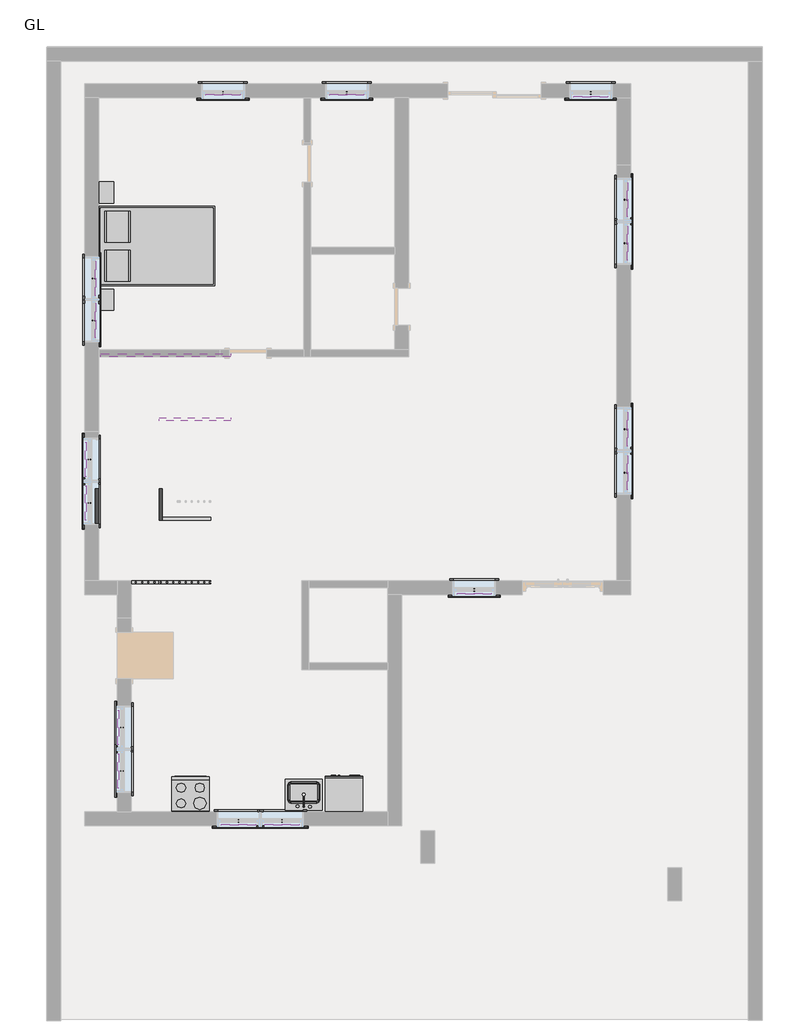
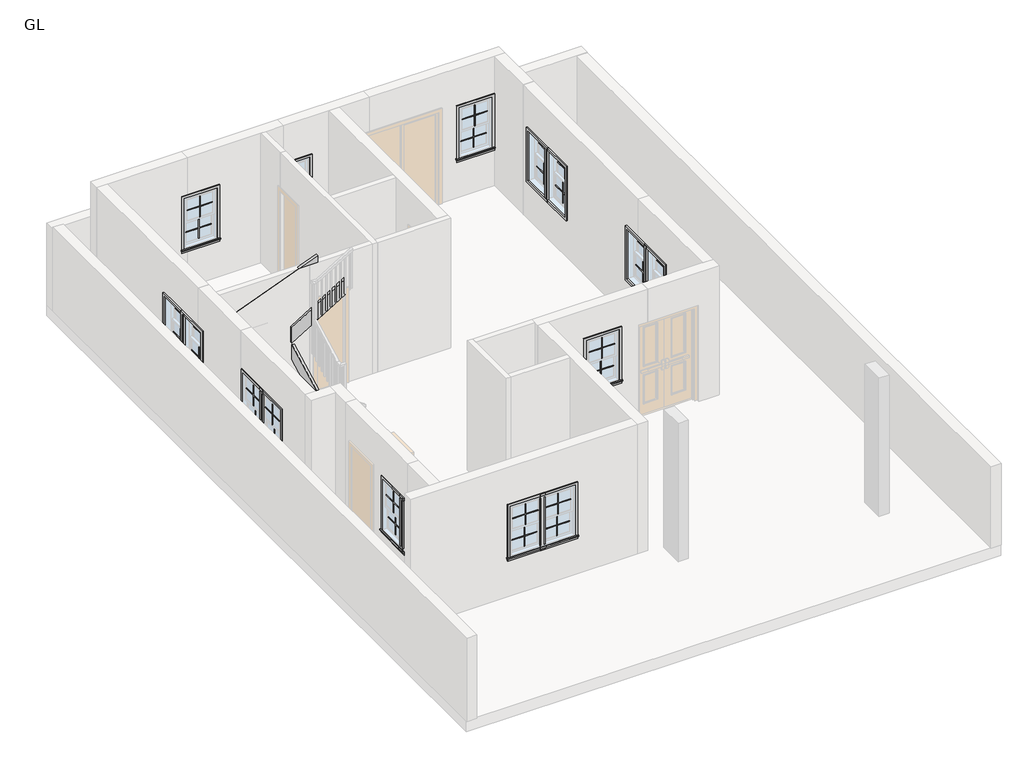
# One storey, part 3 of 3: 66 proxies, 6 members, 1 flow terminal, 1 furniture element.
"""IFC4 building model written with IfcOpenShell, lengths in millimetres."""

from ifc_helpers import new_model, si_unit, frame, origin, place, context, project, spatial, polyline, outline, extrude, transform, mapped, element, save
from components import dishwasher_m_610_x_610_x_860mm_47db8dec, muntin_pattern_2x2_muntin_pattern_2x2_5f474966, range_m_610_x_610mm_88bdc8d1, trim_window_exterior_flat_with_sill_68241f6a, trim_window_interior_flat_picture_frame_d3d93820, m_sink_kitchen_single_760_x_535mm_2_83ebd6f4, modern_beds_1593_1300_x_1900_cc95cf5d

model = new_model("IFC4")

# Units and contexts
model_context = context("Model", 3, world=origin())
ifc_project = project(units=[si_unit("LENGTHUNIT", "METRE", prefix="MILLI")], contexts=[model_context])

# Site, building, storey
site = spatial("IfcSite", under=ifc_project)
building = spatial("IfcBuilding", under=site)
storey = spatial("IfcBuildingStorey", under=building, Name="GL", Elevation=0.0)

# Proxies
placement = place(None, origin())
dishwasher_m_610_x_610_x_860mm_shape = dishwasher_m_610_x_610_x_860mm_47db8dec(model_context)
element("IfcBuildingElementProxy", 1, Name="Dishwasher (M) : 610 x 610 x 860mm", ObjectType="Dishwasher (M) : 610 x 610 x 860mm", at=placement, inside=storey, context=model_context, shape_type="MappedRepresentation", body=[
    mapped(dishwasher_m_610_x_610_x_860mm_shape, transform((-17856.7757002, 1424.9719294, 0.0), x_axis=(-1.0, 0.0, 0.0), y_axis=(0.0, -1.0, 0.0), z_axis=(0.0, 0.0, 1.0))),
])
muntin_pattern_2x2_muntin_pattern_2x2_shape = muntin_pattern_2x2_muntin_pattern_2x2_5f474966(model_context)
element("IfcBuildingElementProxy", 2, Name="Muntin Pattern_2x2 : Muntin Pattern_2x2", ObjectType="Muntin Pattern_2x2 : Muntin Pattern_2x2", at=placement, inside=storey, context=model_context, shape_type="MappedRepresentation", body=[
    mapped(muntin_pattern_2x2_muntin_pattern_2x2_shape, transform((-20215.5750314, 12584.9473147, 1520.825), x_axis=(-1.0, 0.0, 0.0), y_axis=(0.0, -1.0, 0.0), z_axis=(0.0, 0.0, 1.0))),
])
element("IfcBuildingElementProxy", 3, Name="Muntin Pattern_2x2 : Muntin Pattern_2x2", ObjectType="Muntin Pattern_2x2 : Muntin Pattern_2x2", at=placement, inside=storey, context=model_context, shape_type="MappedRepresentation", body=[
    mapped(muntin_pattern_2x2_muntin_pattern_2x2_shape, transform((-20215.5750314, 12629.3973147, 990.6), x_axis=(-1.0, 0.0, 0.0), y_axis=(0.0, -1.0, 0.0), z_axis=(0.0, 0.0, 1.0))),
])
element("IfcBuildingElementProxy", 4, Name="Muntin Pattern_2x2 : Muntin Pattern_2x2", ObjectType="Muntin Pattern_2x2 : Muntin Pattern_2x2", at=placement, inside=storey, context=model_context, shape_type="MappedRepresentation", body=[
    mapped(muntin_pattern_2x2_muntin_pattern_2x2_shape, transform((-14208.4750314, 12584.9473147, 1520.825), x_axis=(-1.0, 0.0, 0.0), y_axis=(0.0, -1.0, 0.0), z_axis=(0.0, 0.0, 1.0))),
])
element("IfcBuildingElementProxy", 5, Name="Muntin Pattern_2x2 : Muntin Pattern_2x2", ObjectType="Muntin Pattern_2x2 : Muntin Pattern_2x2", at=placement, inside=storey, context=model_context, shape_type="MappedRepresentation", body=[
    mapped(muntin_pattern_2x2_muntin_pattern_2x2_shape, transform((-14208.4750314, 12629.3973147, 990.6), x_axis=(-1.0, 0.0, 0.0), y_axis=(0.0, -1.0, 0.0), z_axis=(0.0, 0.0, 1.0))),
])
element("IfcBuildingElementProxy", 6, Name="Muntin Pattern_2x2 : Muntin Pattern_2x2", ObjectType="Muntin Pattern_2x2 : Muntin Pattern_2x2", at=placement, inside=storey, context=model_context, shape_type="MappedRepresentation", body=[
    mapped(muntin_pattern_2x2_muntin_pattern_2x2_shape, transform((-13595.7000314, 10888.3098201, 1520.825), x_axis=(0.0, -1.0, 0.0), y_axis=(1.0, 0.0, 0.0), z_axis=(0.0, 0.0, 1.0))),
])
element("IfcBuildingElementProxy", 7, Name="Muntin Pattern_2x2 : Muntin Pattern_2x2", ObjectType="Muntin Pattern_2x2 : Muntin Pattern_2x2", at=placement, inside=storey, context=model_context, shape_type="MappedRepresentation", body=[
    mapped(muntin_pattern_2x2_muntin_pattern_2x2_shape, transform((-13640.1500314, 10888.3098201, 990.6), x_axis=(0.0, -1.0, 0.0), y_axis=(1.0, 0.0, 0.0), z_axis=(0.0, 0.0, 1.0))),
])
element("IfcBuildingElementProxy", 8, Name="Muntin Pattern_2x2 : Muntin Pattern_2x2", ObjectType="Muntin Pattern_2x2 : Muntin Pattern_2x2", at=placement, inside=storey, context=model_context, shape_type="MappedRepresentation", body=[
    mapped(muntin_pattern_2x2_muntin_pattern_2x2_shape, transform((-13595.7000314, 10177.1098201, 1520.825), x_axis=(0.0, -1.0, 0.0), y_axis=(1.0, 0.0, 0.0), z_axis=(0.0, 0.0, 1.0))),
])
element("IfcBuildingElementProxy", 9, Name="Muntin Pattern_2x2 : Muntin Pattern_2x2", ObjectType="Muntin Pattern_2x2 : Muntin Pattern_2x2", at=placement, inside=storey, context=model_context, shape_type="MappedRepresentation", body=[
    mapped(muntin_pattern_2x2_muntin_pattern_2x2_shape, transform((-13640.1500314, 10177.1098201, 990.6), x_axis=(0.0, -1.0, 0.0), y_axis=(1.0, 0.0, 0.0), z_axis=(0.0, 0.0, 1.0))),
])
element("IfcBuildingElementProxy", 10, Name="Muntin Pattern_2x2 : Muntin Pattern_2x2", ObjectType="Muntin Pattern_2x2 : Muntin Pattern_2x2", at=placement, inside=storey, context=model_context, shape_type="MappedRepresentation", body=[
    mapped(muntin_pattern_2x2_muntin_pattern_2x2_shape, transform((-13595.7000314, 7139.8223646, 1520.825), x_axis=(0.0, -1.0, 0.0), y_axis=(1.0, 0.0, 0.0), z_axis=(0.0, 0.0, 1.0))),
])
element("IfcBuildingElementProxy", 11, Name="Muntin Pattern_2x2 : Muntin Pattern_2x2", ObjectType="Muntin Pattern_2x2 : Muntin Pattern_2x2", at=placement, inside=storey, context=model_context, shape_type="MappedRepresentation", body=[
    mapped(muntin_pattern_2x2_muntin_pattern_2x2_shape, transform((-13640.1500314, 7139.8223646, 990.6), x_axis=(0.0, -1.0, 0.0), y_axis=(1.0, 0.0, 0.0), z_axis=(0.0, 0.0, 1.0))),
])
element("IfcBuildingElementProxy", 12, Name="Muntin Pattern_2x2 : Muntin Pattern_2x2", ObjectType="Muntin Pattern_2x2 : Muntin Pattern_2x2", at=placement, inside=storey, context=model_context, shape_type="MappedRepresentation", body=[
    mapped(muntin_pattern_2x2_muntin_pattern_2x2_shape, transform((-13595.7000314, 6428.6223646, 1520.825), x_axis=(0.0, -1.0, 0.0), y_axis=(1.0, 0.0, 0.0), z_axis=(0.0, 0.0, 1.0))),
])
element("IfcBuildingElementProxy", 13, Name="Muntin Pattern_2x2 : Muntin Pattern_2x2", ObjectType="Muntin Pattern_2x2 : Muntin Pattern_2x2", at=placement, inside=storey, context=model_context, shape_type="MappedRepresentation", body=[
    mapped(muntin_pattern_2x2_muntin_pattern_2x2_shape, transform((-13640.1500314, 6428.6223646, 990.6), x_axis=(0.0, -1.0, 0.0), y_axis=(1.0, 0.0, 0.0), z_axis=(0.0, 0.0, 1.0))),
])
element("IfcBuildingElementProxy", 14, Name="Muntin Pattern_2x2 : Muntin Pattern_2x2", ObjectType="Muntin Pattern_2x2 : Muntin Pattern_2x2", at=placement, inside=storey, context=model_context, shape_type="MappedRepresentation", body=[
    mapped(muntin_pattern_2x2_muntin_pattern_2x2_shape, transform((-19961.4931686, 697.7473646, 1520.825), x_axis=(-1.0, 0.0, 0.0), y_axis=(0.0, -1.0, 0.0), z_axis=(0.0, 0.0, 1.0))),
])
element("IfcBuildingElementProxy", 15, Name="Muntin Pattern_2x2 : Muntin Pattern_2x2", ObjectType="Muntin Pattern_2x2 : Muntin Pattern_2x2", at=placement, inside=storey, context=model_context, shape_type="MappedRepresentation", body=[
    mapped(muntin_pattern_2x2_muntin_pattern_2x2_shape, transform((-19961.4931686, 742.1973646, 990.6), x_axis=(-1.0, 0.0, 0.0), y_axis=(0.0, -1.0, 0.0), z_axis=(0.0, 0.0, 1.0))),
])
element("IfcBuildingElementProxy", 16, Name="Muntin Pattern_2x2 : Muntin Pattern_2x2", ObjectType="Muntin Pattern_2x2 : Muntin Pattern_2x2", at=placement, inside=storey, context=model_context, shape_type="MappedRepresentation", body=[
    mapped(muntin_pattern_2x2_muntin_pattern_2x2_shape, transform((-19250.2931686, 697.7473646, 1520.825), x_axis=(-1.0, 0.0, 0.0), y_axis=(0.0, -1.0, 0.0), z_axis=(0.0, 0.0, 1.0))),
])
element("IfcBuildingElementProxy", 17, Name="Muntin Pattern_2x2 : Muntin Pattern_2x2", ObjectType="Muntin Pattern_2x2 : Muntin Pattern_2x2", at=placement, inside=storey, context=model_context, shape_type="MappedRepresentation", body=[
    mapped(muntin_pattern_2x2_muntin_pattern_2x2_shape, transform((-19250.2931686, 742.1973646, 990.6), x_axis=(-1.0, 0.0, 0.0), y_axis=(0.0, -1.0, 0.0), z_axis=(0.0, 0.0, 1.0))),
])
element("IfcBuildingElementProxy", 18, Name="Muntin Pattern_2x2 : Muntin Pattern_2x2", ObjectType="Muntin Pattern_2x2 : Muntin Pattern_2x2", at=placement, inside=storey, context=model_context, shape_type="MappedRepresentation", body=[
    mapped(muntin_pattern_2x2_muntin_pattern_2x2_shape, transform((-21907.8500314, 2269.3723646, 1520.825), x_axis=(0.0, 1.0, 0.0), y_axis=(-1.0, 0.0, 0.0), z_axis=(0.0, 0.0, 1.0))),
])
element("IfcBuildingElementProxy", 19, Name="Muntin Pattern_2x2 : Muntin Pattern_2x2", ObjectType="Muntin Pattern_2x2 : Muntin Pattern_2x2", at=placement, inside=storey, context=model_context, shape_type="MappedRepresentation", body=[
    mapped(muntin_pattern_2x2_muntin_pattern_2x2_shape, transform((-21863.4000314, 2269.3723646, 990.6), x_axis=(0.0, 1.0, 0.0), y_axis=(-1.0, 0.0, 0.0), z_axis=(0.0, 0.0, 1.0))),
])
element("IfcBuildingElementProxy", 20, Name="Muntin Pattern_2x2 : Muntin Pattern_2x2", ObjectType="Muntin Pattern_2x2 : Muntin Pattern_2x2", at=placement, inside=storey, context=model_context, shape_type="MappedRepresentation", body=[
    mapped(muntin_pattern_2x2_muntin_pattern_2x2_shape, transform((-21907.8500314, 1558.1723646, 1520.825), x_axis=(0.0, 1.0, 0.0), y_axis=(-1.0, 0.0, 0.0), z_axis=(0.0, 0.0, 1.0))),
])
element("IfcBuildingElementProxy", 21, Name="Muntin Pattern_2x2 : Muntin Pattern_2x2", ObjectType="Muntin Pattern_2x2 : Muntin Pattern_2x2", at=placement, inside=storey, context=model_context, shape_type="MappedRepresentation", body=[
    mapped(muntin_pattern_2x2_muntin_pattern_2x2_shape, transform((-21863.4000314, 1558.1723646, 990.6), x_axis=(0.0, 1.0, 0.0), y_axis=(-1.0, 0.0, 0.0), z_axis=(0.0, 0.0, 1.0))),
])
element("IfcBuildingElementProxy", 22, Name="Muntin Pattern_2x2 : Muntin Pattern_2x2", ObjectType="Muntin Pattern_2x2 : Muntin Pattern_2x2", at=placement, inside=storey, context=model_context, shape_type="MappedRepresentation", body=[
    mapped(muntin_pattern_2x2_muntin_pattern_2x2_shape, transform((-22441.2502061, 6644.5223643, 1520.825), x_axis=(0.0, 1.0, 0.0), y_axis=(-1.0, 0.0, 0.0), z_axis=(0.0, 0.0, 1.0))),
])
element("IfcBuildingElementProxy", 23, Name="Muntin Pattern_2x2 : Muntin Pattern_2x2", ObjectType="Muntin Pattern_2x2 : Muntin Pattern_2x2", at=placement, inside=storey, context=model_context, shape_type="MappedRepresentation", body=[
    mapped(muntin_pattern_2x2_muntin_pattern_2x2_shape, transform((-22396.8002061, 6644.5223643, 990.6), x_axis=(0.0, 1.0, 0.0), y_axis=(-1.0, 0.0, 0.0), z_axis=(0.0, 0.0, 1.0))),
])
element("IfcBuildingElementProxy", 24, Name="Muntin Pattern_2x2 : Muntin Pattern_2x2", ObjectType="Muntin Pattern_2x2 : Muntin Pattern_2x2", at=placement, inside=storey, context=model_context, shape_type="MappedRepresentation", body=[
    mapped(muntin_pattern_2x2_muntin_pattern_2x2_shape, transform((-22441.2502061, 5933.3223643, 1520.825), x_axis=(0.0, 1.0, 0.0), y_axis=(-1.0, 0.0, 0.0), z_axis=(0.0, 0.0, 1.0))),
])
element("IfcBuildingElementProxy", 25, Name="Muntin Pattern_2x2 : Muntin Pattern_2x2", ObjectType="Muntin Pattern_2x2 : Muntin Pattern_2x2", at=placement, inside=storey, context=model_context, shape_type="MappedRepresentation", body=[
    mapped(muntin_pattern_2x2_muntin_pattern_2x2_shape, transform((-22396.8002061, 5933.3223643, 990.6), x_axis=(0.0, 1.0, 0.0), y_axis=(-1.0, 0.0, 0.0), z_axis=(0.0, 0.0, 1.0))),
])
element("IfcBuildingElementProxy", 26, Name="Muntin Pattern_2x2 : Muntin Pattern_2x2", ObjectType="Muntin Pattern_2x2 : Muntin Pattern_2x2", at=placement, inside=storey, context=model_context, shape_type="MappedRepresentation", body=[
    mapped(muntin_pattern_2x2_muntin_pattern_2x2_shape, transform((-22282.5000314, 9599.539033, 1520.825), x_axis=(0.0, -1.0, 0.0), y_axis=(1.0, 0.0, 0.0), z_axis=(0.0, 0.0, 1.0))),
])
element("IfcBuildingElementProxy", 27, Name="Muntin Pattern_2x2 : Muntin Pattern_2x2", ObjectType="Muntin Pattern_2x2 : Muntin Pattern_2x2", at=placement, inside=storey, context=model_context, shape_type="MappedRepresentation", body=[
    mapped(muntin_pattern_2x2_muntin_pattern_2x2_shape, transform((-22326.9500314, 9599.539033, 990.6), x_axis=(0.0, -1.0, 0.0), y_axis=(1.0, 0.0, 0.0), z_axis=(0.0, 0.0, 1.0))),
])
element("IfcBuildingElementProxy", 28, Name="Muntin Pattern_2x2 : Muntin Pattern_2x2", ObjectType="Muntin Pattern_2x2 : Muntin Pattern_2x2", at=placement, inside=storey, context=model_context, shape_type="MappedRepresentation", body=[
    mapped(muntin_pattern_2x2_muntin_pattern_2x2_shape, transform((-22282.5000314, 8913.739033, 1520.825), x_axis=(0.0, -1.0, 0.0), y_axis=(1.0, 0.0, 0.0), z_axis=(0.0, 0.0, 1.0))),
])
element("IfcBuildingElementProxy", 29, Name="Muntin Pattern_2x2 : Muntin Pattern_2x2", ObjectType="Muntin Pattern_2x2 : Muntin Pattern_2x2", at=placement, inside=storey, context=model_context, shape_type="MappedRepresentation", body=[
    mapped(muntin_pattern_2x2_muntin_pattern_2x2_shape, transform((-22326.9500314, 8913.739033, 990.6), x_axis=(0.0, -1.0, 0.0), y_axis=(1.0, 0.0, 0.0), z_axis=(0.0, 0.0, 1.0))),
])
element("IfcBuildingElementProxy", 30, Name="Muntin Pattern_2x2 : Muntin Pattern_2x2", ObjectType="Muntin Pattern_2x2 : Muntin Pattern_2x2", at=placement, inside=storey, context=model_context, shape_type="MappedRepresentation", body=[
    mapped(muntin_pattern_2x2_muntin_pattern_2x2_shape, transform((-18193.8494379, 12584.9473147, 1520.825), x_axis=(-1.0, 0.0, 0.0), y_axis=(0.0, -1.0, 0.0), z_axis=(0.0, 0.0, 1.0))),
])
element("IfcBuildingElementProxy", 31, Name="Muntin Pattern_2x2 : Muntin Pattern_2x2", ObjectType="Muntin Pattern_2x2 : Muntin Pattern_2x2", at=placement, inside=storey, context=model_context, shape_type="MappedRepresentation", body=[
    mapped(muntin_pattern_2x2_muntin_pattern_2x2_shape, transform((-18193.8494379, 12629.3973147, 990.6), x_axis=(-1.0, 0.0, 0.0), y_axis=(0.0, -1.0, 0.0), z_axis=(0.0, 0.0, 1.0))),
])
element("IfcBuildingElementProxy", 32, Name="Muntin Pattern_2x2 : Muntin Pattern_2x2", ObjectType="Muntin Pattern_2x2 : Muntin Pattern_2x2", at=placement, inside=storey, context=model_context, shape_type="MappedRepresentation", body=[
    mapped(muntin_pattern_2x2_muntin_pattern_2x2_shape, transform((-16113.4750314, 4469.6473722, 1728.2254923), x_axis=(-1.0, 0.0, 0.0), y_axis=(0.0, -1.0, 0.0), z_axis=(0.0, 0.0, 1.0))),
])
element("IfcBuildingElementProxy", 33, Name="Muntin Pattern_2x2 : Muntin Pattern_2x2", ObjectType="Muntin Pattern_2x2 : Muntin Pattern_2x2", at=placement, inside=storey, context=model_context, shape_type="MappedRepresentation", body=[
    mapped(muntin_pattern_2x2_muntin_pattern_2x2_shape, transform((-16113.4750314, 4514.0973722, 1198.0004923), x_axis=(-1.0, 0.0, 0.0), y_axis=(0.0, -1.0, 0.0), z_axis=(0.0, 0.0, 1.0))),
])
range_m_610_x_610mm_shape = range_m_610_x_610mm_88bdc8d1(model_context)
element("IfcBuildingElementProxy", 34, Name="Range (M) : 610 x 610mm", ObjectType="Range (M) : 610 x 610mm", at=placement, inside=storey, context=model_context, shape_type="MappedRepresentation", body=[
    mapped(range_m_610_x_610mm_shape, transform((-20441.8931686, 1463.3223646, 0.0), x_axis=(-1.0, 0.0, 0.0), y_axis=(0.0, -1.0, 0.0), z_axis=(0.0, 0.0, 1.0))),
])
trim_window_exterior_flat_with_sill_shape = trim_window_exterior_flat_with_sill_68241f6a(model_context)
element("IfcBuildingElementProxy", 35, Name="Trim-Window-Exterior-Flat : with Sill", ObjectType="Trim-Window-Exterior-Flat : with Sill", at=placement, inside=storey, context=model_context, shape_type="MappedRepresentation", body=[
    mapped(trim_window_exterior_flat_with_sill_shape, transform((-20215.5750314, 12550.0223147, 2082.8), x_axis=(1.0, 0.0, 0.0), y_axis=(0.0, 0.0, 1.0), z_axis=(0.0, -1.0, 0.0))),
])
element("IfcBuildingElementProxy", 36, Name="Trim-Window-Exterior-Flat : with Sill", ObjectType="Trim-Window-Exterior-Flat : with Sill", at=placement, inside=storey, context=model_context, shape_type="MappedRepresentation", body=[
    mapped(trim_window_exterior_flat_with_sill_shape, transform((-14208.4750314, 12550.0223147, 2082.8), x_axis=(1.0, 0.0, 0.0), y_axis=(0.0, 0.0, 1.0), z_axis=(0.0, -1.0, 0.0))),
])
element("IfcBuildingElementProxy", 37, Name="Trim-Window-Exterior-Flat : with Sill", ObjectType="Trim-Window-Exterior-Flat : with Sill", at=placement, inside=storey, context=model_context, shape_type="MappedRepresentation", body=[
    mapped(trim_window_exterior_flat_with_sill_shape, transform((-13560.7750314, 10888.3098201, 2082.8), x_axis=(0.0, 1.0, 0.0), y_axis=(0.0, 0.0, 1.0), z_axis=(1.0, 0.0, 0.0))),
])
element("IfcBuildingElementProxy", 38, Name="Trim-Window-Exterior-Flat : with Sill", ObjectType="Trim-Window-Exterior-Flat : with Sill", at=placement, inside=storey, context=model_context, shape_type="MappedRepresentation", body=[
    mapped(trim_window_exterior_flat_with_sill_shape, transform((-13560.7750314, 10177.1098201, 2082.8), x_axis=(0.0, 1.0, 0.0), y_axis=(0.0, 0.0, 1.0), z_axis=(1.0, 0.0, 0.0))),
])
element("IfcBuildingElementProxy", 39, Name="Trim-Window-Exterior-Flat : with Sill", ObjectType="Trim-Window-Exterior-Flat : with Sill", at=placement, inside=storey, context=model_context, shape_type="MappedRepresentation", body=[
    mapped(trim_window_exterior_flat_with_sill_shape, transform((-13560.7750314, 7139.8223646, 2082.8), x_axis=(0.0, 1.0, 0.0), y_axis=(0.0, 0.0, 1.0), z_axis=(1.0, 0.0, 0.0))),
])
element("IfcBuildingElementProxy", 40, Name="Trim-Window-Exterior-Flat : with Sill", ObjectType="Trim-Window-Exterior-Flat : with Sill", at=placement, inside=storey, context=model_context, shape_type="MappedRepresentation", body=[
    mapped(trim_window_exterior_flat_with_sill_shape, transform((-13560.7750314, 6428.6223646, 2082.8), x_axis=(0.0, 1.0, 0.0), y_axis=(0.0, 0.0, 1.0), z_axis=(1.0, 0.0, 0.0))),
])
element("IfcBuildingElementProxy", 41, Name="Trim-Window-Exterior-Flat : with Sill", ObjectType="Trim-Window-Exterior-Flat : with Sill", at=placement, inside=storey, context=model_context, shape_type="MappedRepresentation", body=[
    mapped(trim_window_exterior_flat_with_sill_shape, transform((-19961.4931686, 662.8223646, 2082.8), x_axis=(1.0, 0.0, 0.0), y_axis=(0.0, 0.0, 1.0), z_axis=(0.0, -1.0, 0.0))),
])
element("IfcBuildingElementProxy", 42, Name="Trim-Window-Exterior-Flat : with Sill", ObjectType="Trim-Window-Exterior-Flat : with Sill", at=placement, inside=storey, context=model_context, shape_type="MappedRepresentation", body=[
    mapped(trim_window_exterior_flat_with_sill_shape, transform((-19250.2931686, 662.8223646, 2082.8), x_axis=(1.0, 0.0, 0.0), y_axis=(0.0, 0.0, 1.0), z_axis=(0.0, -1.0, 0.0))),
])
element("IfcBuildingElementProxy", 43, Name="Trim-Window-Exterior-Flat : with Sill", ObjectType="Trim-Window-Exterior-Flat : with Sill", at=placement, inside=storey, context=model_context, shape_type="MappedRepresentation", body=[
    mapped(trim_window_exterior_flat_with_sill_shape, transform((-21942.7750314, 2269.3723646, 2082.8), x_axis=(0.0, -1.0, 0.0), y_axis=(0.0, 0.0, 1.0), z_axis=(-1.0, 0.0, 0.0))),
])
element("IfcBuildingElementProxy", 44, Name="Trim-Window-Exterior-Flat : with Sill", ObjectType="Trim-Window-Exterior-Flat : with Sill", at=placement, inside=storey, context=model_context, shape_type="MappedRepresentation", body=[
    mapped(trim_window_exterior_flat_with_sill_shape, transform((-21942.7750314, 1558.1723646, 2082.8), x_axis=(0.0, -1.0, 0.0), y_axis=(0.0, 0.0, 1.0), z_axis=(-1.0, 0.0, 0.0))),
])
element("IfcBuildingElementProxy", 45, Name="Trim-Window-Exterior-Flat : with Sill", ObjectType="Trim-Window-Exterior-Flat : with Sill", at=placement, inside=storey, context=model_context, shape_type="MappedRepresentation", body=[
    mapped(trim_window_exterior_flat_with_sill_shape, transform((-22476.1752061, 6644.5223643, 2082.8), x_axis=(0.0, -1.0, 0.0), y_axis=(0.0, 0.0, 1.0), z_axis=(-1.0, 0.0, 0.0))),
])
element("IfcBuildingElementProxy", 46, Name="Trim-Window-Exterior-Flat : with Sill", ObjectType="Trim-Window-Exterior-Flat : with Sill", at=placement, inside=storey, context=model_context, shape_type="MappedRepresentation", body=[
    mapped(trim_window_exterior_flat_with_sill_shape, transform((-22476.1752061, 5933.3223643, 2082.8), x_axis=(0.0, -1.0, 0.0), y_axis=(0.0, 0.0, 1.0), z_axis=(-1.0, 0.0, 0.0))),
])
element("IfcBuildingElementProxy", 47, Name="Trim-Window-Exterior-Flat : with Sill", ObjectType="Trim-Window-Exterior-Flat : with Sill", at=placement, inside=storey, context=model_context, shape_type="MappedRepresentation", body=[
    mapped(trim_window_exterior_flat_with_sill_shape, transform((-22247.5750314, 9599.539033, 2082.8), x_axis=(0.0, 1.0, 0.0), y_axis=(0.0, 0.0, 1.0), z_axis=(1.0, 0.0, 0.0))),
])
element("IfcBuildingElementProxy", 48, Name="Trim-Window-Exterior-Flat : with Sill", ObjectType="Trim-Window-Exterior-Flat : with Sill", at=placement, inside=storey, context=model_context, shape_type="MappedRepresentation", body=[
    mapped(trim_window_exterior_flat_with_sill_shape, transform((-22247.5750314, 8913.739033, 2082.8), x_axis=(0.0, 1.0, 0.0), y_axis=(0.0, 0.0, 1.0), z_axis=(1.0, 0.0, 0.0))),
])
element("IfcBuildingElementProxy", 49, Name="Trim-Window-Exterior-Flat : with Sill", ObjectType="Trim-Window-Exterior-Flat : with Sill", at=placement, inside=storey, context=model_context, shape_type="MappedRepresentation", body=[
    mapped(trim_window_exterior_flat_with_sill_shape, transform((-18193.8494379, 12550.0223147, 2082.8), x_axis=(1.0, 0.0, 0.0), y_axis=(0.0, 0.0, 1.0), z_axis=(0.0, -1.0, 0.0))),
])
element("IfcBuildingElementProxy", 50, Name="Trim-Window-Exterior-Flat : with Sill", ObjectType="Trim-Window-Exterior-Flat : with Sill", at=placement, inside=storey, context=model_context, shape_type="MappedRepresentation", body=[
    mapped(trim_window_exterior_flat_with_sill_shape, transform((-16113.4750314, 4434.7223722, 2290.2004923), x_axis=(1.0, 0.0, 0.0), y_axis=(0.0, 0.0, 1.0), z_axis=(0.0, -1.0, 0.0))),
])
trim_window_interior_flat_picture_frame_shape = trim_window_interior_flat_picture_frame_d3d93820(model_context)
element("IfcBuildingElementProxy", 51, Name="Trim-Window-Interior-Flat : Picture Frame", ObjectType="Trim-Window-Interior-Flat : Picture Frame", at=placement, inside=storey, context=model_context, shape_type="MappedRepresentation", body=[
    mapped(trim_window_interior_flat_picture_frame_shape, transform((-20215.5750314, 12778.6223147, 2082.8), x_axis=(-1.0, 0.0, 0.0), y_axis=(0.0, 0.0, 1.0), z_axis=(0.0, 1.0, 0.0))),
])
element("IfcBuildingElementProxy", 52, Name="Trim-Window-Interior-Flat : Picture Frame", ObjectType="Trim-Window-Interior-Flat : Picture Frame", at=placement, inside=storey, context=model_context, shape_type="MappedRepresentation", body=[
    mapped(trim_window_interior_flat_picture_frame_shape, transform((-14208.4750314, 12778.6223147, 2082.8), x_axis=(-1.0, 0.0, 0.0), y_axis=(0.0, 0.0, 1.0), z_axis=(0.0, 1.0, 0.0))),
])
element("IfcBuildingElementProxy", 53, Name="Trim-Window-Interior-Flat : Picture Frame", ObjectType="Trim-Window-Interior-Flat : Picture Frame", at=placement, inside=storey, context=model_context, shape_type="MappedRepresentation", body=[
    mapped(trim_window_interior_flat_picture_frame_shape, transform((-13789.3750314, 10888.3098201, 2082.8), x_axis=(0.0, -1.0, 0.0), y_axis=(0.0, 0.0, 1.0), z_axis=(-1.0, 0.0, 0.0))),
])
element("IfcBuildingElementProxy", 54, Name="Trim-Window-Interior-Flat : Picture Frame", ObjectType="Trim-Window-Interior-Flat : Picture Frame", at=placement, inside=storey, context=model_context, shape_type="MappedRepresentation", body=[
    mapped(trim_window_interior_flat_picture_frame_shape, transform((-13789.3750314, 10177.1098201, 2082.8), x_axis=(0.0, -1.0, 0.0), y_axis=(0.0, 0.0, 1.0), z_axis=(-1.0, 0.0, 0.0))),
])
element("IfcBuildingElementProxy", 55, Name="Trim-Window-Interior-Flat : Picture Frame", ObjectType="Trim-Window-Interior-Flat : Picture Frame", at=placement, inside=storey, context=model_context, shape_type="MappedRepresentation", body=[
    mapped(trim_window_interior_flat_picture_frame_shape, transform((-13789.3750314, 7139.8223646, 2082.8), x_axis=(0.0, -1.0, 0.0), y_axis=(0.0, 0.0, 1.0), z_axis=(-1.0, 0.0, 0.0))),
])
element("IfcBuildingElementProxy", 56, Name="Trim-Window-Interior-Flat : Picture Frame", ObjectType="Trim-Window-Interior-Flat : Picture Frame", at=placement, inside=storey, context=model_context, shape_type="MappedRepresentation", body=[
    mapped(trim_window_interior_flat_picture_frame_shape, transform((-13789.3750314, 6428.6223646, 2082.8), x_axis=(0.0, -1.0, 0.0), y_axis=(0.0, 0.0, 1.0), z_axis=(-1.0, 0.0, 0.0))),
])
element("IfcBuildingElementProxy", 57, Name="Trim-Window-Interior-Flat : Picture Frame", ObjectType="Trim-Window-Interior-Flat : Picture Frame", at=placement, inside=storey, context=model_context, shape_type="MappedRepresentation", body=[
    mapped(trim_window_interior_flat_picture_frame_shape, transform((-19961.4931686, 891.4223646, 2082.8), x_axis=(-1.0, 0.0, 0.0), y_axis=(0.0, 0.0, 1.0), z_axis=(0.0, 1.0, 0.0))),
])
element("IfcBuildingElementProxy", 58, Name="Trim-Window-Interior-Flat : Picture Frame", ObjectType="Trim-Window-Interior-Flat : Picture Frame", at=placement, inside=storey, context=model_context, shape_type="MappedRepresentation", body=[
    mapped(trim_window_interior_flat_picture_frame_shape, transform((-19250.2931686, 891.4223646, 2082.8), x_axis=(-1.0, 0.0, 0.0), y_axis=(0.0, 0.0, 1.0), z_axis=(0.0, 1.0, 0.0))),
])
element("IfcBuildingElementProxy", 59, Name="Trim-Window-Interior-Flat : Picture Frame", ObjectType="Trim-Window-Interior-Flat : Picture Frame", at=placement, inside=storey, context=model_context, shape_type="MappedRepresentation", body=[
    mapped(trim_window_interior_flat_picture_frame_shape, transform((-21714.1750314, 2269.3723646, 2082.8), x_axis=(0.0, 1.0, 0.0), y_axis=(0.0, 0.0, 1.0), z_axis=(1.0, 0.0, 0.0))),
])
element("IfcBuildingElementProxy", 60, Name="Trim-Window-Interior-Flat : Picture Frame", ObjectType="Trim-Window-Interior-Flat : Picture Frame", at=placement, inside=storey, context=model_context, shape_type="MappedRepresentation", body=[
    mapped(trim_window_interior_flat_picture_frame_shape, transform((-21714.1750314, 1558.1723646, 2082.8), x_axis=(0.0, 1.0, 0.0), y_axis=(0.0, 0.0, 1.0), z_axis=(1.0, 0.0, 0.0))),
])
element("IfcBuildingElementProxy", 61, Name="Trim-Window-Interior-Flat : Picture Frame", ObjectType="Trim-Window-Interior-Flat : Picture Frame", at=placement, inside=storey, context=model_context, shape_type="MappedRepresentation", body=[
    mapped(trim_window_interior_flat_picture_frame_shape, transform((-22247.5752061, 6644.5223643, 2082.8), x_axis=(0.0, 1.0, 0.0), y_axis=(0.0, 0.0, 1.0), z_axis=(1.0, 0.0, 0.0))),
])
element("IfcBuildingElementProxy", 62, Name="Trim-Window-Interior-Flat : Picture Frame", ObjectType="Trim-Window-Interior-Flat : Picture Frame", at=placement, inside=storey, context=model_context, shape_type="MappedRepresentation", body=[
    mapped(trim_window_interior_flat_picture_frame_shape, transform((-22247.5752061, 5933.3223643, 2082.8), x_axis=(0.0, 1.0, 0.0), y_axis=(0.0, 0.0, 1.0), z_axis=(1.0, 0.0, 0.0))),
])
element("IfcBuildingElementProxy", 63, Name="Trim-Window-Interior-Flat : Picture Frame", ObjectType="Trim-Window-Interior-Flat : Picture Frame", at=placement, inside=storey, context=model_context, shape_type="MappedRepresentation", body=[
    mapped(trim_window_interior_flat_picture_frame_shape, transform((-22476.1750314, 9599.539033, 2082.8), x_axis=(0.0, -1.0, 0.0), y_axis=(0.0, 0.0, 1.0), z_axis=(-1.0, 0.0, 0.0))),
])
element("IfcBuildingElementProxy", 64, Name="Trim-Window-Interior-Flat : Picture Frame", ObjectType="Trim-Window-Interior-Flat : Picture Frame", at=placement, inside=storey, context=model_context, shape_type="MappedRepresentation", body=[
    mapped(trim_window_interior_flat_picture_frame_shape, transform((-22476.1750314, 8913.739033, 2082.8), x_axis=(0.0, -1.0, 0.0), y_axis=(0.0, 0.0, 1.0), z_axis=(-1.0, 0.0, 0.0))),
])
element("IfcBuildingElementProxy", 65, Name="Trim-Window-Interior-Flat : Picture Frame", ObjectType="Trim-Window-Interior-Flat : Picture Frame", at=placement, inside=storey, context=model_context, shape_type="MappedRepresentation", body=[
    mapped(trim_window_interior_flat_picture_frame_shape, transform((-18193.8494379, 12778.6223147, 2082.8), x_axis=(-1.0, 0.0, 0.0), y_axis=(0.0, 0.0, 1.0), z_axis=(0.0, 1.0, 0.0))),
])
element("IfcBuildingElementProxy", 66, Name="Trim-Window-Interior-Flat : Picture Frame", ObjectType="Trim-Window-Interior-Flat : Picture Frame", at=placement, inside=storey, context=model_context, shape_type="MappedRepresentation", body=[
    mapped(trim_window_interior_flat_picture_frame_shape, transform((-16113.4750314, 4663.3223722, 2290.2004923), x_axis=(-1.0, 0.0, 0.0), y_axis=(0.0, 0.0, 1.0), z_axis=(0.0, 1.0, 0.0))),
])

# Flow terminal
m_sink_kitchen_single_760_x_535mm_2_shape = m_sink_kitchen_single_760_x_535mm_2_83ebd6f4(model_context)
element("IfcFlowTerminal", 67, ObjectType="M_Sink Kitchen-Single : 760 x 535mm 2", at=placement, inside=storey, context=model_context, shape_type="MappedRepresentation", body=[
    mapped(m_sink_kitchen_single_760_x_535mm_2_shape, transform((-18912.5824092, 1173.3677657, 0.0), x_axis=(1.0, 0.0, 0.0), y_axis=(0.0, 1.0, 0.0), z_axis=(0.0, 0.0, 1.0))),
])

# Furniture
modern_beds_1593_1300_x_1900_shape = modern_beds_1593_1300_x_1900_cc95cf5d(model_context)
element("IfcFurniture", 68, ObjectType="Modern_Beds_1593 : 1300 x 1900", at=placement, inside=storey, context=model_context, shape_type="MappedRepresentation", body=[
    mapped(modern_beds_1593_1300_x_1900_shape, transform((-21532.0045396, 9789.8241008, 0.0), x_axis=(0.0, 1.0, 0.0), y_axis=(-1.0, 0.0, 0.0), z_axis=(0.0, 0.0, 1.0))),
])

# Members
element("IfcMember", 69, ObjectType="Stringer - 2\" Width", at=placement, inside=storey, context=model_context, shape_type="SweptSolid", body=[
    extrude(outline(polyline([(130.5252239, -20418.7750314), (452.8815263, -20418.7750314), (746.9746925, -21273.045657), (746.9746925, -22209.4139641), (130.5252239, -20418.7750314)])), frame((0.0, 4612.5223646, 0.0), z_axis=(0.0, 1.0, 0.0), x_axis=(0.0, 0.0, 1.0)), (0.0, 0.0, 1.0), 50.8),
])
element("IfcMember", 70, ObjectType="Stringer - 2\" Width", at=placement, inside=storey, context=model_context, shape_type="SweptSolid", body=[
    extrude(outline(polyline([(4688.0958922, 760.1121693), (7646.6888829, 2329.0629977), (8297.2722107, 2329.0629977), (5338.67922, 760.1121693), (4688.0958922, 760.1121693)])), frame((-22298.3752061, 0.0, 0.0), z_axis=(1.0, 0.0, 0.0), x_axis=(0.0, 1.0, 0.0)), (0.0, 0.0, 1.0), 50.8),
])
element("IfcMember", 71, ObjectType="Stringer - 2\" Width", at=placement, inside=storey, context=model_context, shape_type="SweptSolid", body=[
    extrude(outline(polyline([(2341.604746, -21363.7701417), (2830.7206787, -20088.5750314), (3157.1726538, -20088.5750314), (2341.604746, -22214.8770766), (2341.604746, -21363.7701417)])), frame((0.0, 8320.9223646, 0.0), z_axis=(0.0, 1.0, 0.0), x_axis=(0.0, 0.0, 1.0)), (0.0, 0.0, 1.0), 50.8),
])
element("IfcMember", 72, ObjectType="Stringer - 2\" Width", at=placement, inside=storey, context=model_context, shape_type="SweptSolid", body=[
    extrude(outline(polyline([(31.5282995, -20418.7750314), (392.8106437, -20418.7750314), (893.883371, -21206.1750314), (532.6010268, -21206.1750314), (31.5282995, -20418.7750314)])), frame((0.0, 5653.9223646, 0.0), z_axis=(0.0, 1.0, 0.0), x_axis=(0.0, 0.0, 1.0)), (0.0, 0.0, 1.0), 50.8),
])
element("IfcMember", 73, ObjectType="Stringer - 2\" Width", at=placement, inside=storey, context=model_context, shape_type="SweptSolid", body=[
    extrude(outline(polyline([(5653.9223646, 927.2865642), (5653.9223646, 1272.2928743), (7279.5223646, 2134.3534804), (7279.5223646, 1789.3471702), (5653.9223646, 927.2865642)])), frame((-21256.9750314, 0.0, 0.0), z_axis=(1.0, 0.0, 0.0), x_axis=(0.0, 1.0, 0.0)), (0.0, 0.0, 1.0), 50.8),
])
element("IfcMember", 74, ObjectType="Stringer - 2\" Width", at=placement, inside=storey, context=model_context, shape_type="SweptSolid", body=[
    extrude(outline(polyline([(2524.6057942, -21256.9750314), (2166.3538932, -21256.9750314), (2888.0127167, -20088.5750314), (3246.2646178, -20088.5750314), (2524.6057942, -21256.9750314)])), frame((0.0, 7279.5223646, 0.0), z_axis=(0.0, 1.0, 0.0), x_axis=(0.0, 0.0, 1.0)), (0.0, 0.0, 1.0), 50.8),
])

save(model, "model.ifc")

# Revit data of these elements
# Type "Dishwasher (M) : 610 x 610 x 860mm"
#   Label = "DW"
#   Depth = 2' - 0.01575"
#   Height = 2' - 9.85827"
#   Width = 2' - 0.01575"
#   Dishwasher Material = Metal - Paint Finish - Ivory,Glossy
#   Panel Face Material = Plastic - Black
#   Default Elevation = 0
# Type "Muntin Pattern_2x2 : Muntin Pattern_2x2"
#   Width [instance default] = 4' - 0"
#   Thickness = 0' - 0 1/2"
#   Height [instance default] = 4' - 0"
#   Distance = 0' - 0 3/4"
#   Interior Material [instance default] = none
#   Exterior Material [instance default] = none
#   Default Elevation = 0
# Type "Range (M) : 610 x 610mm"
#   Depth = 2' - 0.01575"
#   Width = 2' - 0.01575"
#   Burner Material = Metal - Chrome
#   Range Material = Metal - Painted Finish - Ivory,Matte
#   Default Elevation = 0
#   Assembly Code = ""
# Type "Trim-Window-Exterior-Flat : with Sill"
#   Trim Width = 0' - 2 1/4"
#   Trim Thickness_Picture Frame = 0' - 1 1/4"
#   Trim Thickness_with Sill = 0' - 0 3/4"
#   Sill Thickness = 0' - 1 1/4"
#   Opening Width [instance default] = 2' - 0"
#   Opening Height [instance default] = 3' - 0"
#   Default Elevation = 4' - 0"
#   Sill = yes
#   Picture Frame = no
#   Trim Material [instance default] = none
# Type "Trim-Window-Interior-Flat : Picture Frame"
#   Trim Thickness_Picture Frame = 0' - 1 1/4"
#   Trim Width = 0' - 2 1/4"
#   Trim Thickness_with Sill = 0' - 0 3/4"
#   Sill Thickness = 0' - 1 1/4"
#   Opening Width [instance default] = 2' - 0"
#   Opening Height [instance default] = 3' - 0"
#   Default Elevation = 4' - 0"
#   Sill = no
#   Picture Frame = yes
#   Trim Material [instance default] = none
# Type "M_Sink Kitchen-Single : 760 x 535mm 2"
#   Counter Height = 3' - 0.22047"
#   Depth = 1' - 7.68504"
#   Width = 1' - 11.62205"
#   Fixture Material = Metal - Steel, Polished
#   Sink Material = Metal - Steel, Polished
#   Default Elevation = 0
#   Assembly Code = ""
# Type "Modern_Beds_1593 : 1300 x 1900"
#   Length = 6' - 2.80315"
#   Width = 4' - 3.1811"
#   Frame Material = Bed-Wood
#   Mattress Material = Bed-Cover
#   Default Elevation = 0
# Element 1 (IfcBuildingElementProxy, "Dishwasher (M) : 610 x 610 x 860mm")
#   Phase Created = New Construction
#   Materials on its faces: "Metal - Paint Finish - Ivory,Glossy", "Plastic - Black"
# Elements 2, 3, 4, 5, 6, 7, 8, 9, 10, 11, 12, 13, 14, 15, 16, 17, 18, 19, 20, 21, 22, 23, 24, 25, 26, 27, 28, 29, 30, 31, 32, 33 (IfcBuildingElementProxy, "Muntin Pattern_2x2 : Muntin Pattern_2x2")
#   Width = 1' - 10"
#   Height = 1' - 7 1/8"
#   Interior Material = Wood - Stained
#   Exterior Material = Clad - White
#   Phase Created = New Construction
#   Materials on its faces: "Clad - White", "Wood - Stained"
# Element 34 (IfcBuildingElementProxy, "Range (M) : 610 x 610mm")
#   Phase Created = New Construction
#   Materials on its faces: "Metal - Painted Finish - Ivory,Matte", "Metal - Chrome", "Glass"
# Elements 35, 36, 37, 38, 39, 40, 41, 42, 43, 44, 45, 46, 47, 48, 49, 50 (IfcBuildingElementProxy, "Trim-Window-Exterior-Flat : with Sill")
#   Opening Width = 2' - 4"
#   Opening Height = 3' - 10"
#   Trim Material = Clad - White
#   Phase Created = New Construction
#   Materials on its faces: "Clad - White"
# Elements 51, 52, 53, 54, 55, 56, 57, 58, 59, 60, 61, 62, 63, 64, 65, 66 (IfcBuildingElementProxy, "Trim-Window-Interior-Flat : Picture Frame")
#   Opening Width = 2' - 4"
#   Opening Height = 3' - 10"
#   Trim Material = Wood - Stained
#   Phase Created = New Construction
#   Materials on its faces: "Wood - Stained"
# Element 67 (IfcFlowTerminal, "M_Sink Kitchen-Single : 760 x 535mm 2")
#   Mark = "1"
#   Phase Created = New Construction
#   Materials on its faces: "Metal - Steel, Polished"
# Element 68 (IfcFurniture, "Modern_Beds_1593 : 1300 x 1900")
#   Phase Created = New Construction
#   Materials on its faces: "Bed-Metal", "Bed-Cover", "Bed-Wood"
# Elements 69, 70, 71, 72, 73, 74 (IfcMember, "Stringer - 2\" Width")
#   Phase Created = New Construction
# Materials
#   "Metal - Paint Finish - Ivory,Glossy": colour RGB 247 247 239, transparency 0
#   "Plastic - Black": colour RGB 0 0 0, transparency 0.7
#   "Metal - Chrome": colour RGB 17 17 17, transparency 0
#   "Metal - Painted Finish - Ivory,Matte": colour RGB 247 247 239, transparency 0
#   "Metal - Steel, Polished": class "Metal", colour RGB 192 192 192, transparency 0
#   "Bed-Wood": colour RGB 224 178 126, transparency 0
#   "Bed-Cover": colour RGB 255 255 255, transparency 0
#   "Clad - White": class "Wood", colour RGB 242 242 238, transparency 0, Cost = 0
#   "Wood - Stained": class "Wood", colour RGB 224 178 126, transparency 0, Cost = 0
#   "Glass": class "Glass", colour RGB 0 128 192, transparency 0.75, Description = "Soda Lime Glass", Cost = 0
#   "Bed-Metal": colour RGB 247 247 247, transparency 0
